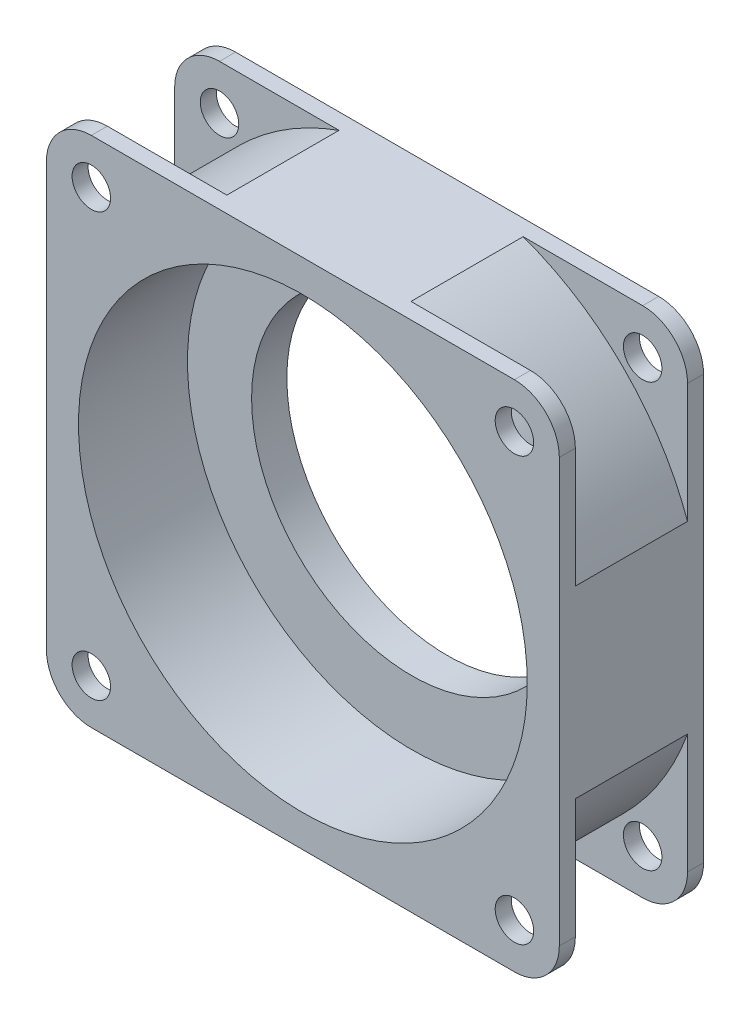
ISO-10303-21;
HEADER;
FILE_DESCRIPTION(('STEP AP214'),'2;1');
FILE_NAME('part.step','',(''),(''),'','','');
FILE_SCHEMA(('AUTOMOTIVE_DESIGN { 1 0 10303 214 1 1 1 1 }'));
ENDSEC;
DATA;
#1=APPLICATION_CONTEXT('core data for automotive mechanical design processes');
#2=APPLICATION_PROTOCOL_DEFINITION('international standard','automotive_design',2000,#1);
#3=PRODUCT_CONTEXT('',#1,'mechanical');
#4=PRODUCT('Part','Part','',(#3));
#5=PRODUCT_RELATED_PRODUCT_CATEGORY('part','',(#4));
#6=PRODUCT_DEFINITION_FORMATION('','',#4);
#7=PRODUCT_DEFINITION_CONTEXT('part definition',#1,'design');
#8=PRODUCT_DEFINITION('design','',#6,#7);
#9=PRODUCT_DEFINITION_SHAPE('','',#8);
#10=(LENGTH_UNIT() NAMED_UNIT(*) SI_UNIT(.MILLI.,.METRE.));
#11=(NAMED_UNIT(*) PLANE_ANGLE_UNIT() SI_UNIT($,.RADIAN.));
#12=(NAMED_UNIT(*) SI_UNIT($,.STERADIAN.) SOLID_ANGLE_UNIT());
#13=UNCERTAINTY_MEASURE_WITH_UNIT(LENGTH_MEASURE(1.E-05),#10,'distance_accuracy_value','');
#14=(GEOMETRIC_REPRESENTATION_CONTEXT(3) GLOBAL_UNCERTAINTY_ASSIGNED_CONTEXT((#13)) GLOBAL_UNIT_ASSIGNED_CONTEXT((#10,
#11,#12)) REPRESENTATION_CONTEXT('',''));
#15=CARTESIAN_POINT('',(0.,0.,0.));
#16=DIRECTION('',(0.,0.,1.));
#17=DIRECTION('',(1.,0.,0.));
#18=AXIS2_PLACEMENT_3D('',#15,#16,#17);
#19=CARTESIAN_POINT('',(0.,0.,20.));
#20=DIRECTION('',(0.,0.,1.));
#21=DIRECTION('',(1.,0.,0.));
#22=AXIS2_PLACEMENT_3D('',#19,#20,#21);
#23=PLANE('',#22);
#24=CARTESIAN_POINT('',(-33.,73.,20.));
#25=DIRECTION('',(0.,0.,1.));
#26=DIRECTION('',(1.,0.,0.));
#27=AXIS2_PLACEMENT_3D('',#24,#25,#26);
#28=CIRCLE('',#27,3.);
#29=CARTESIAN_POINT('',(-30.,73.,20.));
#30=VERTEX_POINT('',#29);
#31=EDGE_CURVE('E381',#30,#30,#28,.T.);
#32=ORIENTED_EDGE('',*,*,#31,.T.);
#33=EDGE_LOOP('',(#32));
#34=FACE_BOUND('',#33,.T.);
#35=DIRECTION('',(-1.,0.,0.));
#36=VECTOR('',#35,1.);
#37=CARTESIAN_POINT('',(0.,80.,20.));
#38=LINE('',#37,#36);
#39=CARTESIAN_POINT('',(-14.3614066163451,80.,20.));
#40=VERTEX_POINT('',#39);
#41=CARTESIAN_POINT('',(-33.,80.,20.));
#42=VERTEX_POINT('',#41);
#43=EDGE_CURVE('E262',#40,#42,#38,.T.);
#44=ORIENTED_EDGE('',*,*,#43,.F.);
#45=CARTESIAN_POINT('',(0.,40.,20.));
#46=DIRECTION('',(0.,0.,1.));
#47=DIRECTION('',(1.,0.,0.));
#48=AXIS2_PLACEMENT_3D('',#45,#46,#47);
#49=CIRCLE('',#48,42.5);
#50=CARTESIAN_POINT('',(-40.,54.3614066163451,20.));
#51=VERTEX_POINT('',#50);
#52=EDGE_CURVE('E249',#40,#51,#49,.T.);
#53=ORIENTED_EDGE('',*,*,#52,.T.);
#54=DIRECTION('',(0.,-1.,0.));
#55=VECTOR('',#54,1.);
#56=CARTESIAN_POINT('',(-40.,0.,20.));
#57=LINE('',#56,#55);
#58=CARTESIAN_POINT('',(-40.,72.9999999999999,20.));
#59=VERTEX_POINT('',#58);
#60=EDGE_CURVE('E268',#59,#51,#57,.T.);
#61=ORIENTED_EDGE('',*,*,#60,.F.);
#62=CARTESIAN_POINT('',(-33.,73.,20.));
#63=DIRECTION('',(0.,0.,1.));
#64=DIRECTION('',(1.,0.,0.));
#65=AXIS2_PLACEMENT_3D('',#62,#63,#64);
#66=CIRCLE('',#65,7.);
#67=EDGE_CURVE('E263',#42,#59,#66,.T.);
#68=ORIENTED_EDGE('',*,*,#67,.F.);
#69=EDGE_LOOP('',(#44,#53,#61,#68));
#70=FACE_BOUND('',#69,.T.);
#71=ADVANCED_FACE('F50',(#34,#70),#23,.F.);
#72=CARTESIAN_POINT('',(33.,73.,20.));
#73=DIRECTION('',(0.,0.,1.));
#74=DIRECTION('',(1.,0.,0.));
#75=AXIS2_PLACEMENT_3D('',#72,#73,#74);
#76=CIRCLE('',#75,3.00000000000001);
#77=CARTESIAN_POINT('',(36.,73.,20.));
#78=VERTEX_POINT('',#77);
#79=EDGE_CURVE('E389',#78,#78,#76,.T.);
#80=ORIENTED_EDGE('',*,*,#79,.T.);
#81=EDGE_LOOP('',(#80));
#82=FACE_BOUND('',#81,.T.);
#83=DIRECTION('',(0.,1.,0.));
#84=VECTOR('',#83,1.);
#85=CARTESIAN_POINT('',(40.,0.,20.));
#86=LINE('',#85,#84);
#87=CARTESIAN_POINT('',(40.,54.3614066163451,20.));
#88=VERTEX_POINT('',#87);
#89=CARTESIAN_POINT('',(40.,72.9999999999999,20.));
#90=VERTEX_POINT('',#89);
#91=EDGE_CURVE('E259',#88,#90,#86,.T.);
#92=ORIENTED_EDGE('',*,*,#91,.F.);
#93=CARTESIAN_POINT('',(0.,40.,20.));
#94=DIRECTION('',(0.,0.,1.));
#95=DIRECTION('',(1.,0.,0.));
#96=AXIS2_PLACEMENT_3D('',#93,#94,#95);
#97=CIRCLE('',#96,42.5);
#98=CARTESIAN_POINT('',(14.3614066163451,80.,20.));
#99=VERTEX_POINT('',#98);
#100=EDGE_CURVE('E250',#88,#99,#97,.T.);
#101=ORIENTED_EDGE('',*,*,#100,.T.);
#102=CARTESIAN_POINT('',(33.,80.,20.));
#103=VERTEX_POINT('',#102);
#104=EDGE_CURVE('E265',#103,#99,#38,.T.);
#105=ORIENTED_EDGE('',*,*,#104,.F.);
#106=CARTESIAN_POINT('',(33.,73.,20.));
#107=DIRECTION('',(0.,0.,1.));
#108=DIRECTION('',(1.,0.,0.));
#109=AXIS2_PLACEMENT_3D('',#106,#107,#108);
#110=CIRCLE('',#109,7.);
#111=EDGE_CURVE('E260',#90,#103,#110,.T.);
#112=ORIENTED_EDGE('',*,*,#111,.F.);
#113=EDGE_LOOP('',(#92,#101,#105,#112));
#114=FACE_BOUND('',#113,.T.);
#115=ADVANCED_FACE('F494',(#82,#114),#23,.F.);
#116=CARTESIAN_POINT('',(33.,7.,20.));
#117=DIRECTION('',(0.,0.,1.));
#118=DIRECTION('',(1.,0.,0.));
#119=AXIS2_PLACEMENT_3D('',#116,#117,#118);
#120=CIRCLE('',#119,3.);
#121=CARTESIAN_POINT('',(36.,7.,20.));
#122=VERTEX_POINT('',#121);
#123=EDGE_CURVE('E395',#122,#122,#120,.T.);
#124=ORIENTED_EDGE('',*,*,#123,.T.);
#125=EDGE_LOOP('',(#124));
#126=FACE_BOUND('',#125,.T.);
#127=DIRECTION('',(1.,0.,0.));
#128=VECTOR('',#127,1.);
#129=CARTESIAN_POINT('',(0.,0.,20.));
#130=LINE('',#129,#128);
#131=CARTESIAN_POINT('',(14.3614066163451,0.,20.));
#132=VERTEX_POINT('',#131);
#133=CARTESIAN_POINT('',(33.,0.,20.));
#134=VERTEX_POINT('',#133);
#135=EDGE_CURVE('E273',#132,#134,#130,.T.);
#136=ORIENTED_EDGE('',*,*,#135,.F.);
#137=CARTESIAN_POINT('',(0.,40.,20.));
#138=DIRECTION('',(0.,0.,1.));
#139=DIRECTION('',(1.,0.,0.));
#140=AXIS2_PLACEMENT_3D('',#137,#138,#139);
#141=CIRCLE('',#140,42.5);
#142=CARTESIAN_POINT('',(40.,25.6385933836549,20.));
#143=VERTEX_POINT('',#142);
#144=EDGE_CURVE('E243',#132,#143,#141,.T.);
#145=ORIENTED_EDGE('',*,*,#144,.T.);
#146=CARTESIAN_POINT('',(40.,7.00000000000005,20.));
#147=VERTEX_POINT('',#146);
#148=EDGE_CURVE('E251',#147,#143,#86,.T.);
#149=ORIENTED_EDGE('',*,*,#148,.F.);
#150=CARTESIAN_POINT('',(33.,7.,20.));
#151=DIRECTION('',(0.,0.,1.));
#152=DIRECTION('',(1.,0.,0.));
#153=AXIS2_PLACEMENT_3D('',#150,#151,#152);
#154=CIRCLE('',#153,7.);
#155=EDGE_CURVE('E276',#134,#147,#154,.T.);
#156=ORIENTED_EDGE('',*,*,#155,.F.);
#157=EDGE_LOOP('',(#136,#145,#149,#156));
#158=FACE_BOUND('',#157,.T.);
#159=ADVANCED_FACE('F439',(#126,#158),#23,.F.);
#160=CARTESIAN_POINT('',(33.,7.,20.));
#161=DIRECTION('',(0.,0.,1.));
#162=DIRECTION('',(1.,0.,0.));
#163=AXIS2_PLACEMENT_3D('',#160,#161,#162);
#164=CYLINDRICAL_SURFACE('',#163,7.);
#165=CARTESIAN_POINT('',(33.,7.,22.5));
#166=DIRECTION('',(0.,0.,1.));
#167=DIRECTION('',(1.,0.,0.));
#168=AXIS2_PLACEMENT_3D('',#165,#166,#167);
#169=CIRCLE('',#168,7.);
#170=CARTESIAN_POINT('',(33.,0.,22.5));
#171=VERTEX_POINT('',#170);
#172=CARTESIAN_POINT('',(40.,7.00000000000005,22.5));
#173=VERTEX_POINT('',#172);
#174=EDGE_CURVE('E299',#171,#173,#169,.T.);
#175=ORIENTED_EDGE('',*,*,#174,.F.);
#176=DIRECTION('',(0.,0.,1.));
#177=VECTOR('',#176,1.);
#178=CARTESIAN_POINT('',(33.,0.,20.));
#179=LINE('',#178,#177);
#180=EDGE_CURVE('E304',#134,#171,#179,.T.);
#181=ORIENTED_EDGE('',*,*,#180,.F.);
#182=ORIENTED_EDGE('',*,*,#155,.T.);
#183=DIRECTION('',(0.,0.,1.));
#184=VECTOR('',#183,1.);
#185=CARTESIAN_POINT('',(40.,7.00000000000005,20.));
#186=LINE('',#185,#184);
#187=EDGE_CURVE('E305',#147,#173,#186,.T.);
#188=ORIENTED_EDGE('',*,*,#187,.T.);
#189=EDGE_LOOP('',(#175,#181,#182,#188));
#190=FACE_BOUND('',#189,.T.);
#191=ADVANCED_FACE('F443',(#190),#164,.T.);
#192=CARTESIAN_POINT('',(-33.,7.,20.));
#193=DIRECTION('',(0.,0.,1.));
#194=DIRECTION('',(1.,0.,0.));
#195=AXIS2_PLACEMENT_3D('',#192,#193,#194);
#196=CYLINDRICAL_SURFACE('',#195,7.);
#197=CARTESIAN_POINT('',(-33.,7.,22.5));
#198=DIRECTION('',(0.,0.,1.));
#199=DIRECTION('',(1.,0.,0.));
#200=AXIS2_PLACEMENT_3D('',#197,#198,#199);
#201=CIRCLE('',#200,7.);
#202=CARTESIAN_POINT('',(-33.,0.,22.5));
#203=VERTEX_POINT('',#202);
#204=CARTESIAN_POINT('',(-40.,7.00000000000005,22.5));
#205=VERTEX_POINT('',#204);
#206=EDGE_CURVE('E295',#203,#205,#201,.F.);
#207=ORIENTED_EDGE('',*,*,#206,.T.);
#208=DIRECTION('',(0.,0.,1.));
#209=VECTOR('',#208,1.);
#210=CARTESIAN_POINT('',(-40.,7.00000000000005,20.));
#211=LINE('',#210,#209);
#212=CARTESIAN_POINT('',(-40.,7.00000000000005,20.));
#213=VERTEX_POINT('',#212);
#214=EDGE_CURVE('E309',#213,#205,#211,.T.);
#215=ORIENTED_EDGE('',*,*,#214,.F.);
#216=CARTESIAN_POINT('',(-33.,7.,20.));
#217=DIRECTION('',(0.,0.,1.));
#218=DIRECTION('',(1.,0.,0.));
#219=AXIS2_PLACEMENT_3D('',#216,#217,#218);
#220=CIRCLE('',#219,7.);
#221=CARTESIAN_POINT('',(-33.,0.,20.));
#222=VERTEX_POINT('',#221);
#223=EDGE_CURVE('E275',#222,#213,#220,.F.);
#224=ORIENTED_EDGE('',*,*,#223,.F.);
#225=DIRECTION('',(0.,0.,1.));
#226=VECTOR('',#225,1.);
#227=CARTESIAN_POINT('',(-33.,0.,20.));
#228=LINE('',#227,#226);
#229=EDGE_CURVE('E308',#222,#203,#228,.T.);
#230=ORIENTED_EDGE('',*,*,#229,.T.);
#231=EDGE_LOOP('',(#207,#215,#224,#230));
#232=FACE_BOUND('',#231,.T.);
#233=ADVANCED_FACE('F451',(#232),#196,.T.);
#234=CARTESIAN_POINT('',(-33.,73.,20.));
#235=DIRECTION('',(0.,0.,1.));
#236=DIRECTION('',(1.,0.,0.));
#237=AXIS2_PLACEMENT_3D('',#234,#235,#236);
#238=CYLINDRICAL_SURFACE('',#237,7.);
#239=CARTESIAN_POINT('',(-33.,73.,22.5));
#240=DIRECTION('',(0.,0.,1.));
#241=DIRECTION('',(1.,0.,0.));
#242=AXIS2_PLACEMENT_3D('',#239,#240,#241);
#243=CIRCLE('',#242,7.);
#244=CARTESIAN_POINT('',(-33.,80.,22.5));
#245=VERTEX_POINT('',#244);
#246=CARTESIAN_POINT('',(-40.,72.9999999999999,22.5));
#247=VERTEX_POINT('',#246);
#248=EDGE_CURVE('E288',#245,#247,#243,.T.);
#249=ORIENTED_EDGE('',*,*,#248,.F.);
#250=DIRECTION('',(0.,0.,1.));
#251=VECTOR('',#250,1.);
#252=CARTESIAN_POINT('',(-33.,80.,20.));
#253=LINE('',#252,#251);
#254=EDGE_CURVE('E314',#42,#245,#253,.T.);
#255=ORIENTED_EDGE('',*,*,#254,.F.);
#256=ORIENTED_EDGE('',*,*,#67,.T.);
#257=DIRECTION('',(0.,0.,1.));
#258=VECTOR('',#257,1.);
#259=CARTESIAN_POINT('',(-40.,72.9999999999999,20.));
#260=LINE('',#259,#258);
#261=EDGE_CURVE('E312',#59,#247,#260,.T.);
#262=ORIENTED_EDGE('',*,*,#261,.T.);
#263=EDGE_LOOP('',(#249,#255,#256,#262));
#264=FACE_BOUND('',#263,.T.);
#265=ADVANCED_FACE('F517',(#264),#238,.T.);
#266=CARTESIAN_POINT('',(33.,73.,20.));
#267=DIRECTION('',(0.,0.,1.));
#268=DIRECTION('',(1.,0.,0.));
#269=AXIS2_PLACEMENT_3D('',#266,#267,#268);
#270=CYLINDRICAL_SURFACE('',#269,7.);
#271=CARTESIAN_POINT('',(33.,73.,22.5));
#272=DIRECTION('',(0.,0.,1.));
#273=DIRECTION('',(1.,0.,0.));
#274=AXIS2_PLACEMENT_3D('',#271,#272,#273);
#275=CIRCLE('',#274,7.);
#276=CARTESIAN_POINT('',(40.,72.9999999999999,22.5));
#277=VERTEX_POINT('',#276);
#278=CARTESIAN_POINT('',(33.,80.,22.5));
#279=VERTEX_POINT('',#278);
#280=EDGE_CURVE('E281',#277,#279,#275,.T.);
#281=ORIENTED_EDGE('',*,*,#280,.F.);
#282=DIRECTION('',(0.,0.,1.));
#283=VECTOR('',#282,1.);
#284=CARTESIAN_POINT('',(40.,72.9999999999999,20.));
#285=LINE('',#284,#283);
#286=EDGE_CURVE('E285',#90,#277,#285,.T.);
#287=ORIENTED_EDGE('',*,*,#286,.F.);
#288=ORIENTED_EDGE('',*,*,#111,.T.);
#289=DIRECTION('',(0.,0.,1.));
#290=VECTOR('',#289,1.);
#291=CARTESIAN_POINT('',(33.,80.,20.));
#292=LINE('',#291,#290);
#293=EDGE_CURVE('E319',#103,#279,#292,.T.);
#294=ORIENTED_EDGE('',*,*,#293,.T.);
#295=EDGE_LOOP('',(#281,#287,#288,#294));
#296=FACE_BOUND('',#295,.T.);
#297=ADVANCED_FACE('F506',(#296),#270,.T.);
#298=CARTESIAN_POINT('',(-33.,7.,20.));
#299=DIRECTION('',(0.,0.,1.));
#300=DIRECTION('',(1.,0.,0.));
#301=AXIS2_PLACEMENT_3D('',#298,#299,#300);
#302=CIRCLE('',#301,3.);
#303=CARTESIAN_POINT('',(-30.,7.,20.));
#304=VERTEX_POINT('',#303);
#305=EDGE_CURVE('E410',#304,#304,#302,.T.);
#306=ORIENTED_EDGE('',*,*,#305,.T.);
#307=EDGE_LOOP('',(#306));
#308=FACE_BOUND('',#307,.T.);
#309=CARTESIAN_POINT('',(-40.,25.6385933836549,20.));
#310=VERTEX_POINT('',#309);
#311=EDGE_CURVE('E267',#310,#213,#57,.T.);
#312=ORIENTED_EDGE('',*,*,#311,.F.);
#313=CARTESIAN_POINT('',(0.,40.,20.));
#314=DIRECTION('',(0.,0.,1.));
#315=DIRECTION('',(1.,0.,0.));
#316=AXIS2_PLACEMENT_3D('',#313,#314,#315);
#317=CIRCLE('',#316,42.5);
#318=CARTESIAN_POINT('',(-14.3614066163451,0.,20.));
#319=VERTEX_POINT('',#318);
#320=EDGE_CURVE('E233',#310,#319,#317,.T.);
#321=ORIENTED_EDGE('',*,*,#320,.T.);
#322=EDGE_CURVE('E277',#222,#319,#130,.T.);
#323=ORIENTED_EDGE('',*,*,#322,.F.);
#324=ORIENTED_EDGE('',*,*,#223,.T.);
#325=EDGE_LOOP('',(#312,#321,#323,#324));
#326=FACE_BOUND('',#325,.T.);
#327=ADVANCED_FACE('F460',(#308,#326),#23,.F.);
#328=CARTESIAN_POINT('',(0.,40.,22.5));
#329=DIRECTION('',(0.,0.,1.));
#330=DIRECTION('',(1.,0.,0.));
#331=AXIS2_PLACEMENT_3D('',#328,#329,#330);
#332=PLANE('',#331);
#333=CARTESIAN_POINT('',(33.,73.,22.5));
#334=DIRECTION('',(0.,0.,1.));
#335=DIRECTION('',(1.,0.,0.));
#336=AXIS2_PLACEMENT_3D('',#333,#334,#335);
#337=CIRCLE('',#336,3.00000000000001);
#338=CARTESIAN_POINT('',(36.,73.,22.5));
#339=VERTEX_POINT('',#338);
#340=EDGE_CURVE('E880',#339,#339,#337,.T.);
#341=ORIENTED_EDGE('',*,*,#340,.F.);
#342=EDGE_LOOP('',(#341));
#343=FACE_BOUND('',#342,.T.);
#344=CARTESIAN_POINT('',(-33.,7.,22.5));
#345=DIRECTION('',(0.,0.,1.));
#346=DIRECTION('',(1.,0.,0.));
#347=AXIS2_PLACEMENT_3D('',#344,#345,#346);
#348=CIRCLE('',#347,3.);
#349=CARTESIAN_POINT('',(-30.,7.,22.5));
#350=VERTEX_POINT('',#349);
#351=EDGE_CURVE('E879',#350,#350,#348,.T.);
#352=ORIENTED_EDGE('',*,*,#351,.F.);
#353=EDGE_LOOP('',(#352));
#354=FACE_BOUND('',#353,.T.);
#355=CARTESIAN_POINT('',(33.,7.,22.5));
#356=DIRECTION('',(0.,0.,1.));
#357=DIRECTION('',(1.,0.,0.));
#358=AXIS2_PLACEMENT_3D('',#355,#356,#357);
#359=CIRCLE('',#358,3.);
#360=CARTESIAN_POINT('',(36.,7.,22.5));
#361=VERTEX_POINT('',#360);
#362=EDGE_CURVE('E882',#361,#361,#359,.T.);
#363=ORIENTED_EDGE('',*,*,#362,.F.);
#364=EDGE_LOOP('',(#363));
#365=FACE_BOUND('',#364,.T.);
#366=CARTESIAN_POINT('',(-33.,73.,22.5));
#367=DIRECTION('',(0.,0.,1.));
#368=DIRECTION('',(1.,0.,0.));
#369=AXIS2_PLACEMENT_3D('',#366,#367,#368);
#370=CIRCLE('',#369,3.);
#371=CARTESIAN_POINT('',(-30.,73.,22.5));
#372=VERTEX_POINT('',#371);
#373=EDGE_CURVE('E379',#372,#372,#370,.T.);
#374=ORIENTED_EDGE('',*,*,#373,.F.);
#375=EDGE_LOOP('',(#374));
#376=FACE_BOUND('',#375,.T.);
#377=CARTESIAN_POINT('',(0.,40.,22.5));
#378=DIRECTION('',(0.,0.,1.));
#379=DIRECTION('',(1.,0.,0.));
#380=AXIS2_PLACEMENT_3D('',#377,#378,#379);
#381=CIRCLE('',#380,35.);
#382=CARTESIAN_POINT('',(35.,40.,22.5));
#383=VERTEX_POINT('',#382);
#384=EDGE_CURVE('E372',#383,#383,#381,.T.);
#385=ORIENTED_EDGE('',*,*,#384,.F.);
#386=EDGE_LOOP('',(#385));
#387=FACE_BOUND('',#386,.T.);
#388=DIRECTION('',(1.,0.,0.));
#389=VECTOR('',#388,1.);
#390=CARTESIAN_POINT('',(0.,0.,22.5));
#391=LINE('',#390,#389);
#392=EDGE_CURVE('E300',#203,#171,#391,.T.);
#393=ORIENTED_EDGE('',*,*,#392,.T.);
#394=ORIENTED_EDGE('',*,*,#174,.T.);
#395=DIRECTION('',(0.,1.,0.));
#396=VECTOR('',#395,1.);
#397=CARTESIAN_POINT('',(40.,0.,22.5));
#398=LINE('',#397,#396);
#399=EDGE_CURVE('E254',#173,#277,#398,.T.);
#400=ORIENTED_EDGE('',*,*,#399,.T.);
#401=ORIENTED_EDGE('',*,*,#280,.T.);
#402=DIRECTION('',(-1.,0.,0.));
#403=VECTOR('',#402,1.);
#404=CARTESIAN_POINT('',(0.,80.,22.5));
#405=LINE('',#404,#403);
#406=EDGE_CURVE('E290',#279,#245,#405,.T.);
#407=ORIENTED_EDGE('',*,*,#406,.T.);
#408=ORIENTED_EDGE('',*,*,#248,.T.);
#409=DIRECTION('',(0.,-1.,0.));
#410=VECTOR('',#409,1.);
#411=CARTESIAN_POINT('',(-40.,0.,22.5));
#412=LINE('',#411,#410);
#413=EDGE_CURVE('E292',#247,#205,#412,.T.);
#414=ORIENTED_EDGE('',*,*,#413,.T.);
#415=ORIENTED_EDGE('',*,*,#206,.F.);
#416=EDGE_LOOP('',(#393,#394,#400,#401,#407,#408,#414,#415));
#417=FACE_BOUND('',#416,.T.);
#418=ADVANCED_FACE('F448',(#343,#354,#365,#376,#387,#417),#332,.T.);
#419=CARTESIAN_POINT('',(0.,40.,2.5));
#420=DIRECTION('',(0.,0.,1.));
#421=DIRECTION('',(1.,0.,0.));
#422=AXIS2_PLACEMENT_3D('',#419,#420,#421);
#423=CYLINDRICAL_SURFACE('',#422,42.5);
#424=ORIENTED_EDGE('',*,*,#52,.F.);
#425=DIRECTION('',(0.,0.,1.));
#426=VECTOR('',#425,1.);
#427=CARTESIAN_POINT('',(-14.3614066163451,80.,2.5));
#428=LINE('',#427,#426);
#429=CARTESIAN_POINT('',(-14.3614066163451,80.,2.5));
#430=VERTEX_POINT('',#429);
#431=EDGE_CURVE('E242',#430,#40,#428,.T.);
#432=ORIENTED_EDGE('',*,*,#431,.F.);
#433=CARTESIAN_POINT('',(0.,40.,2.5));
#434=DIRECTION('',(0.,0.,1.));
#435=DIRECTION('',(1.,0.,0.));
#436=AXIS2_PLACEMENT_3D('',#433,#434,#435);
#437=CIRCLE('',#436,42.5);
#438=CARTESIAN_POINT('',(-40.,54.3614066163451,2.5));
#439=VERTEX_POINT('',#438);
#440=EDGE_CURVE('E66',#430,#439,#437,.T.);
#441=ORIENTED_EDGE('',*,*,#440,.T.);
#442=DIRECTION('',(0.,0.,1.));
#443=VECTOR('',#442,1.);
#444=CARTESIAN_POINT('',(-40.,54.3614066163451,2.5));
#445=LINE('',#444,#443);
#446=EDGE_CURVE('E234',#439,#51,#445,.T.);
#447=ORIENTED_EDGE('',*,*,#446,.T.);
#448=EDGE_LOOP('',(#424,#432,#441,#447));
#449=FACE_BOUND('',#448,.T.);
#450=ADVANCED_FACE('F489',(#449),#423,.T.);
#451=CARTESIAN_POINT('',(0.,40.,2.5));
#452=DIRECTION('',(0.,0.,1.));
#453=DIRECTION('',(1.,0.,0.));
#454=AXIS2_PLACEMENT_3D('',#451,#452,#453);
#455=CYLINDRICAL_SURFACE('',#454,42.5);
#456=ORIENTED_EDGE('',*,*,#100,.F.);
#457=DIRECTION('',(0.,0.,1.));
#458=VECTOR('',#457,1.);
#459=CARTESIAN_POINT('',(40.,54.3614066163451,2.5));
#460=LINE('',#459,#458);
#461=CARTESIAN_POINT('',(40.,54.3614066163451,2.5));
#462=VERTEX_POINT('',#461);
#463=EDGE_CURVE('E428',#462,#88,#460,.T.);
#464=ORIENTED_EDGE('',*,*,#463,.F.);
#465=CARTESIAN_POINT('',(0.,40.,2.5));
#466=DIRECTION('',(0.,0.,1.));
#467=DIRECTION('',(1.,0.,0.));
#468=AXIS2_PLACEMENT_3D('',#465,#466,#467);
#469=CIRCLE('',#468,42.5);
#470=CARTESIAN_POINT('',(14.3614066163451,80.,2.5));
#471=VERTEX_POINT('',#470);
#472=EDGE_CURVE('E238',#462,#471,#469,.T.);
#473=ORIENTED_EDGE('',*,*,#472,.T.);
#474=DIRECTION('',(0.,0.,1.));
#475=VECTOR('',#474,1.);
#476=CARTESIAN_POINT('',(14.3614066163451,80.,2.5));
#477=LINE('',#476,#475);
#478=EDGE_CURVE('E425',#471,#99,#477,.T.);
#479=ORIENTED_EDGE('',*,*,#478,.T.);
#480=EDGE_LOOP('',(#456,#464,#473,#479));
#481=FACE_BOUND('',#480,.T.);
#482=ADVANCED_FACE('F485',(#481),#455,.T.);
#483=CARTESIAN_POINT('',(0.,40.,2.5));
#484=DIRECTION('',(0.,0.,1.));
#485=DIRECTION('',(1.,0.,0.));
#486=AXIS2_PLACEMENT_3D('',#483,#484,#485);
#487=CYLINDRICAL_SURFACE('',#486,42.5);
#488=ORIENTED_EDGE('',*,*,#144,.F.);
#489=DIRECTION('',(0.,0.,1.));
#490=VECTOR('',#489,1.);
#491=CARTESIAN_POINT('',(14.3614066163451,0.,2.5));
#492=LINE('',#491,#490);
#493=CARTESIAN_POINT('',(14.3614066163451,0.,2.5));
#494=VERTEX_POINT('',#493);
#495=EDGE_CURVE('E236',#494,#132,#492,.T.);
#496=ORIENTED_EDGE('',*,*,#495,.F.);
#497=CARTESIAN_POINT('',(0.,40.,2.5));
#498=DIRECTION('',(0.,0.,1.));
#499=DIRECTION('',(1.,0.,0.));
#500=AXIS2_PLACEMENT_3D('',#497,#498,#499);
#501=CIRCLE('',#500,42.5);
#502=CARTESIAN_POINT('',(40.,25.6385933836549,2.5));
#503=VERTEX_POINT('',#502);
#504=EDGE_CURVE('E227',#494,#503,#501,.T.);
#505=ORIENTED_EDGE('',*,*,#504,.T.);
#506=DIRECTION('',(0.,0.,1.));
#507=VECTOR('',#506,1.);
#508=CARTESIAN_POINT('',(40.,25.6385933836549,2.5));
#509=LINE('',#508,#507);
#510=EDGE_CURVE('E429',#503,#143,#509,.T.);
#511=ORIENTED_EDGE('',*,*,#510,.T.);
#512=EDGE_LOOP('',(#488,#496,#505,#511));
#513=FACE_BOUND('',#512,.T.);
#514=ADVANCED_FACE('F478',(#513),#487,.T.);
#515=CARTESIAN_POINT('',(0.,40.,2.5));
#516=DIRECTION('',(0.,0.,1.));
#517=DIRECTION('',(1.,0.,0.));
#518=AXIS2_PLACEMENT_3D('',#515,#516,#517);
#519=CYLINDRICAL_SURFACE('',#518,42.5);
#520=ORIENTED_EDGE('',*,*,#320,.F.);
#521=DIRECTION('',(0.,0.,1.));
#522=VECTOR('',#521,1.);
#523=CARTESIAN_POINT('',(-40.,25.6385933836549,2.5));
#524=LINE('',#523,#522);
#525=CARTESIAN_POINT('',(-40.,25.6385933836549,2.5));
#526=VERTEX_POINT('',#525);
#527=EDGE_CURVE('E215',#526,#310,#524,.T.);
#528=ORIENTED_EDGE('',*,*,#527,.F.);
#529=CARTESIAN_POINT('',(0.,40.,2.5));
#530=DIRECTION('',(0.,0.,1.));
#531=DIRECTION('',(1.,0.,0.));
#532=AXIS2_PLACEMENT_3D('',#529,#530,#531);
#533=CIRCLE('',#532,42.5);
#534=CARTESIAN_POINT('',(-14.3614066163451,0.,2.5));
#535=VERTEX_POINT('',#534);
#536=EDGE_CURVE('E221',#526,#535,#533,.T.);
#537=ORIENTED_EDGE('',*,*,#536,.T.);
#538=DIRECTION('',(0.,0.,1.));
#539=VECTOR('',#538,1.);
#540=CARTESIAN_POINT('',(-14.3614066163451,0.,2.5));
#541=LINE('',#540,#539);
#542=EDGE_CURVE('E231',#535,#319,#541,.T.);
#543=ORIENTED_EDGE('',*,*,#542,.T.);
#544=EDGE_LOOP('',(#520,#528,#537,#543));
#545=FACE_BOUND('',#544,.T.);
#546=ADVANCED_FACE('F230',(#545),#519,.T.);
#547=CARTESIAN_POINT('',(33.,73.,2.5));
#548=DIRECTION('',(0.,0.,-1.));
#549=DIRECTION('',(-1.,0.,0.));
#550=AXIS2_PLACEMENT_3D('',#547,#548,#549);
#551=CYLINDRICAL_SURFACE('',#550,7.);
#552=CARTESIAN_POINT('',(33.,73.,0.));
#553=DIRECTION('',(0.,0.,1.));
#554=DIRECTION('',(1.,0.,0.));
#555=AXIS2_PLACEMENT_3D('',#552,#553,#554);
#556=CIRCLE('',#555,7.);
#557=CARTESIAN_POINT('',(40.,73.,0.));
#558=VERTEX_POINT('',#557);
#559=CARTESIAN_POINT('',(33.,80.,0.));
#560=VERTEX_POINT('',#559);
#561=EDGE_CURVE('E344',#558,#560,#556,.T.);
#562=ORIENTED_EDGE('',*,*,#561,.T.);
#563=DIRECTION('',(0.,0.,-1.));
#564=VECTOR('',#563,1.);
#565=CARTESIAN_POINT('',(33.,80.,2.5));
#566=LINE('',#565,#564);
#567=CARTESIAN_POINT('',(33.,80.,2.5));
#568=VERTEX_POINT('',#567);
#569=EDGE_CURVE('E361',#568,#560,#566,.T.);
#570=ORIENTED_EDGE('',*,*,#569,.F.);
#571=CARTESIAN_POINT('',(33.,73.,2.5));
#572=DIRECTION('',(0.,0.,1.));
#573=DIRECTION('',(1.,0.,0.));
#574=AXIS2_PLACEMENT_3D('',#571,#572,#573);
#575=CIRCLE('',#574,7.);
#576=CARTESIAN_POINT('',(40.,73.,2.5));
#577=VERTEX_POINT('',#576);
#578=EDGE_CURVE('E326',#577,#568,#575,.T.);
#579=ORIENTED_EDGE('',*,*,#578,.F.);
#580=DIRECTION('',(0.,0.,-1.));
#581=VECTOR('',#580,1.);
#582=CARTESIAN_POINT('',(40.,73.,2.5));
#583=LINE('',#582,#581);
#584=EDGE_CURVE('E366',#577,#558,#583,.T.);
#585=ORIENTED_EDGE('',*,*,#584,.T.);
#586=EDGE_LOOP('',(#562,#570,#579,#585));
#587=FACE_BOUND('',#586,.T.);
#588=ADVANCED_FACE('F486',(#587),#551,.T.);
#589=CARTESIAN_POINT('',(33.,7.,2.5));
#590=DIRECTION('',(0.,0.,-1.));
#591=DIRECTION('',(-1.,0.,0.));
#592=AXIS2_PLACEMENT_3D('',#589,#590,#591);
#593=CYLINDRICAL_SURFACE('',#592,7.);
#594=CARTESIAN_POINT('',(33.,7.,0.));
#595=DIRECTION('',(0.,0.,1.));
#596=DIRECTION('',(1.,0.,0.));
#597=AXIS2_PLACEMENT_3D('',#594,#595,#596);
#598=CIRCLE('',#597,7.);
#599=CARTESIAN_POINT('',(33.,0.,0.));
#600=VERTEX_POINT('',#599);
#601=CARTESIAN_POINT('',(40.,7.,0.));
#602=VERTEX_POINT('',#601);
#603=EDGE_CURVE('E339',#600,#602,#598,.T.);
#604=ORIENTED_EDGE('',*,*,#603,.T.);
#605=DIRECTION('',(0.,0.,-1.));
#606=VECTOR('',#605,1.);
#607=CARTESIAN_POINT('',(40.,7.,2.5));
#608=LINE('',#607,#606);
#609=CARTESIAN_POINT('',(40.,7.,2.5));
#610=VERTEX_POINT('',#609);
#611=EDGE_CURVE('E57',#610,#602,#608,.T.);
#612=ORIENTED_EDGE('',*,*,#611,.F.);
#613=CARTESIAN_POINT('',(33.,7.,2.5));
#614=DIRECTION('',(0.,0.,1.));
#615=DIRECTION('',(1.,0.,0.));
#616=AXIS2_PLACEMENT_3D('',#613,#614,#615);
#617=CIRCLE('',#616,7.);
#618=CARTESIAN_POINT('',(33.,0.,2.5));
#619=VERTEX_POINT('',#618);
#620=EDGE_CURVE('E324',#619,#610,#617,.T.);
#621=ORIENTED_EDGE('',*,*,#620,.F.);
#622=DIRECTION('',(0.,0.,-1.));
#623=VECTOR('',#622,1.);
#624=CARTESIAN_POINT('',(33.,0.,2.5));
#625=LINE('',#624,#623);
#626=EDGE_CURVE('E11',#619,#600,#625,.T.);
#627=ORIENTED_EDGE('',*,*,#626,.T.);
#628=EDGE_LOOP('',(#604,#612,#621,#627));
#629=FACE_BOUND('',#628,.T.);
#630=ADVANCED_FACE('F472',(#629),#593,.T.);
#631=CARTESIAN_POINT('',(-33.,73.,2.5));
#632=DIRECTION('',(0.,0.,-1.));
#633=DIRECTION('',(-1.,0.,0.));
#634=AXIS2_PLACEMENT_3D('',#631,#632,#633);
#635=CYLINDRICAL_SURFACE('',#634,7.);
#636=CARTESIAN_POINT('',(-33.,73.,0.));
#637=DIRECTION('',(0.,0.,1.));
#638=DIRECTION('',(-1.,0.,0.));
#639=AXIS2_PLACEMENT_3D('',#636,#637,#638);
#640=CIRCLE('',#639,7.);
#641=CARTESIAN_POINT('',(-33.,80.,0.));
#642=VERTEX_POINT('',#641);
#643=CARTESIAN_POINT('',(-40.,73.,0.));
#644=VERTEX_POINT('',#643);
#645=EDGE_CURVE('E350',#642,#644,#640,.T.);
#646=ORIENTED_EDGE('',*,*,#645,.T.);
#647=DIRECTION('',(0.,0.,-1.));
#648=VECTOR('',#647,1.);
#649=CARTESIAN_POINT('',(-40.,73.,2.5));
#650=LINE('',#649,#648);
#651=CARTESIAN_POINT('',(-40.,73.,2.5));
#652=VERTEX_POINT('',#651);
#653=EDGE_CURVE('E357',#652,#644,#650,.T.);
#654=ORIENTED_EDGE('',*,*,#653,.F.);
#655=CARTESIAN_POINT('',(-33.,73.,2.5));
#656=DIRECTION('',(0.,0.,1.));
#657=DIRECTION('',(-1.,0.,0.));
#658=AXIS2_PLACEMENT_3D('',#655,#656,#657);
#659=CIRCLE('',#658,7.);
#660=CARTESIAN_POINT('',(-33.,80.,2.5));
#661=VERTEX_POINT('',#660);
#662=EDGE_CURVE('E219',#661,#652,#659,.T.);
#663=ORIENTED_EDGE('',*,*,#662,.F.);
#664=DIRECTION('',(0.,0.,-1.));
#665=VECTOR('',#664,1.);
#666=CARTESIAN_POINT('',(-33.,80.,2.5));
#667=LINE('',#666,#665);
#668=EDGE_CURVE('E359',#661,#642,#667,.T.);
#669=ORIENTED_EDGE('',*,*,#668,.T.);
#670=EDGE_LOOP('',(#646,#654,#663,#669));
#671=FACE_BOUND('',#670,.T.);
#672=ADVANCED_FACE('F625',(#671),#635,.T.);
#673=CARTESIAN_POINT('',(-33.,7.,2.5));
#674=DIRECTION('',(0.,0.,-1.));
#675=DIRECTION('',(-1.,0.,0.));
#676=AXIS2_PLACEMENT_3D('',#673,#674,#675);
#677=CYLINDRICAL_SURFACE('',#676,7.);
#678=CARTESIAN_POINT('',(-33.,7.,0.));
#679=DIRECTION('',(0.,0.,1.));
#680=DIRECTION('',(-1.,0.,0.));
#681=AXIS2_PLACEMENT_3D('',#678,#679,#680);
#682=CIRCLE('',#681,7.);
#683=CARTESIAN_POINT('',(-40.,7.00000000000005,0.));
#684=VERTEX_POINT('',#683);
#685=CARTESIAN_POINT('',(-33.,0.,0.));
#686=VERTEX_POINT('',#685);
#687=EDGE_CURVE('E351',#684,#686,#682,.T.);
#688=ORIENTED_EDGE('',*,*,#687,.T.);
#689=DIRECTION('',(0.,0.,-1.));
#690=VECTOR('',#689,1.);
#691=CARTESIAN_POINT('',(-33.,0.,2.5));
#692=LINE('',#691,#690);
#693=CARTESIAN_POINT('',(-33.,0.,2.5));
#694=VERTEX_POINT('',#693);
#695=EDGE_CURVE('E340',#694,#686,#692,.T.);
#696=ORIENTED_EDGE('',*,*,#695,.F.);
#697=CARTESIAN_POINT('',(-33.,7.,2.5));
#698=DIRECTION('',(0.,0.,1.));
#699=DIRECTION('',(-1.,0.,0.));
#700=AXIS2_PLACEMENT_3D('',#697,#698,#699);
#701=CIRCLE('',#700,7.);
#702=CARTESIAN_POINT('',(-40.,7.00000000000005,2.5));
#703=VERTEX_POINT('',#702);
#704=EDGE_CURVE('E334',#703,#694,#701,.T.);
#705=ORIENTED_EDGE('',*,*,#704,.F.);
#706=DIRECTION('',(0.,0.,-1.));
#707=VECTOR('',#706,1.);
#708=CARTESIAN_POINT('',(-40.,7.00000000000005,2.5));
#709=LINE('',#708,#707);
#710=EDGE_CURVE('E213',#703,#684,#709,.T.);
#711=ORIENTED_EDGE('',*,*,#710,.T.);
#712=EDGE_LOOP('',(#688,#696,#705,#711));
#713=FACE_BOUND('',#712,.T.);
#714=ADVANCED_FACE('F458',(#713),#677,.T.);
#715=CARTESIAN_POINT('',(33.,7.,0.));
#716=DIRECTION('',(0.,0.,1.));
#717=DIRECTION('',(1.,0.,0.));
#718=AXIS2_PLACEMENT_3D('',#715,#716,#717);
#719=PLANE('',#718);
#720=CARTESIAN_POINT('',(33.,73.,0.));
#721=DIRECTION('',(0.,0.,1.));
#722=DIRECTION('',(1.,0.,0.));
#723=AXIS2_PLACEMENT_3D('',#720,#721,#722);
#724=CIRCLE('',#723,3.00000000000001);
#725=CARTESIAN_POINT('',(36.,73.,0.));
#726=VERTEX_POINT('',#725);
#727=EDGE_CURVE('E384',#726,#726,#724,.T.);
#728=ORIENTED_EDGE('',*,*,#727,.T.);
#729=EDGE_LOOP('',(#728));
#730=FACE_BOUND('',#729,.T.);
#731=CARTESIAN_POINT('',(-33.,7.,0.));
#732=DIRECTION('',(0.,0.,1.));
#733=DIRECTION('',(1.,0.,0.));
#734=AXIS2_PLACEMENT_3D('',#731,#732,#733);
#735=CIRCLE('',#734,3.);
#736=CARTESIAN_POINT('',(-30.,7.,0.));
#737=VERTEX_POINT('',#736);
#738=EDGE_CURVE('E404',#737,#737,#735,.T.);
#739=ORIENTED_EDGE('',*,*,#738,.T.);
#740=EDGE_LOOP('',(#739));
#741=FACE_BOUND('',#740,.T.);
#742=CARTESIAN_POINT('',(33.,7.,0.));
#743=DIRECTION('',(0.,0.,1.));
#744=DIRECTION('',(1.,0.,0.));
#745=AXIS2_PLACEMENT_3D('',#742,#743,#744);
#746=CIRCLE('',#745,3.);
#747=CARTESIAN_POINT('',(36.,7.,0.));
#748=VERTEX_POINT('',#747);
#749=EDGE_CURVE('E390',#748,#748,#746,.T.);
#750=ORIENTED_EDGE('',*,*,#749,.T.);
#751=EDGE_LOOP('',(#750));
#752=FACE_BOUND('',#751,.T.);
#753=CARTESIAN_POINT('',(-33.,73.,0.));
#754=DIRECTION('',(0.,0.,1.));
#755=DIRECTION('',(1.,0.,0.));
#756=AXIS2_PLACEMENT_3D('',#753,#754,#755);
#757=CIRCLE('',#756,3.);
#758=CARTESIAN_POINT('',(-30.,73.,0.));
#759=VERTEX_POINT('',#758);
#760=EDGE_CURVE('E378',#759,#759,#757,.T.);
#761=ORIENTED_EDGE('',*,*,#760,.T.);
#762=EDGE_LOOP('',(#761));
#763=FACE_BOUND('',#762,.T.);
#764=CARTESIAN_POINT('',(0.,40.,0.));
#765=DIRECTION('',(0.,0.,1.));
#766=DIRECTION('',(1.,0.,0.));
#767=AXIS2_PLACEMENT_3D('',#764,#765,#766);
#768=CIRCLE('',#767,25.);
#769=CARTESIAN_POINT('',(25.,40.,0.));
#770=VERTEX_POINT('',#769);
#771=EDGE_CURVE('E371',#770,#770,#768,.T.);
#772=ORIENTED_EDGE('',*,*,#771,.T.);
#773=EDGE_LOOP('',(#772));
#774=FACE_BOUND('',#773,.T.);
#775=DIRECTION('',(1.,0.,0.));
#776=VECTOR('',#775,1.);
#777=CARTESIAN_POINT('',(0.,0.,0.));
#778=LINE('',#777,#776);
#779=EDGE_CURVE('E302',#686,#600,#778,.T.);
#780=ORIENTED_EDGE('',*,*,#779,.F.);
#781=ORIENTED_EDGE('',*,*,#687,.F.);
#782=DIRECTION('',(0.,-1.,0.));
#783=VECTOR('',#782,1.);
#784=CARTESIAN_POINT('',(-40.,73.,0.));
#785=LINE('',#784,#783);
#786=EDGE_CURVE('E346',#644,#684,#785,.T.);
#787=ORIENTED_EDGE('',*,*,#786,.F.);
#788=ORIENTED_EDGE('',*,*,#645,.F.);
#789=DIRECTION('',(-1.,0.,0.));
#790=VECTOR('',#789,1.);
#791=CARTESIAN_POINT('',(33.,80.,0.));
#792=LINE('',#791,#790);
#793=EDGE_CURVE('E343',#560,#642,#792,.T.);
#794=ORIENTED_EDGE('',*,*,#793,.F.);
#795=ORIENTED_EDGE('',*,*,#561,.F.);
#796=DIRECTION('',(0.,1.,0.));
#797=VECTOR('',#796,1.);
#798=CARTESIAN_POINT('',(40.,7.00000000000005,0.));
#799=LINE('',#798,#797);
#800=EDGE_CURVE('E342',#602,#558,#799,.T.);
#801=ORIENTED_EDGE('',*,*,#800,.F.);
#802=ORIENTED_EDGE('',*,*,#603,.F.);
#803=EDGE_LOOP('',(#780,#781,#787,#788,#794,#795,#801,#802));
#804=FACE_BOUND('',#803,.T.);
#805=ADVANCED_FACE('F463',(#730,#741,#752,#763,#774,#804),#719,.F.);
#806=CARTESIAN_POINT('',(-40.,73.,2.5));
#807=DIRECTION('',(1.,0.,0.));
#808=DIRECTION('',(0.,0.,-1.));
#809=AXIS2_PLACEMENT_3D('',#806,#807,#808);
#810=PLANE('',#809);
#811=ORIENTED_EDGE('',*,*,#786,.T.);
#812=ORIENTED_EDGE('',*,*,#710,.F.);
#813=DIRECTION('',(0.,-1.,0.));
#814=VECTOR('',#813,1.);
#815=CARTESIAN_POINT('',(-40.,73.,2.5));
#816=LINE('',#815,#814);
#817=EDGE_CURVE('E206',#526,#703,#816,.T.);
#818=ORIENTED_EDGE('',*,*,#817,.F.);
#819=ORIENTED_EDGE('',*,*,#527,.T.);
#820=ORIENTED_EDGE('',*,*,#311,.T.);
#821=ORIENTED_EDGE('',*,*,#214,.T.);
#822=ORIENTED_EDGE('',*,*,#413,.F.);
#823=ORIENTED_EDGE('',*,*,#261,.F.);
#824=ORIENTED_EDGE('',*,*,#60,.T.);
#825=ORIENTED_EDGE('',*,*,#446,.F.);
#826=EDGE_CURVE('E61',#652,#439,#816,.T.);
#827=ORIENTED_EDGE('',*,*,#826,.F.);
#828=ORIENTED_EDGE('',*,*,#653,.T.);
#829=EDGE_LOOP('',(#811,#812,#818,#819,#820,#821,#822,#823,#824,#825,#827,#828));
#830=FACE_BOUND('',#829,.T.);
#831=ADVANCED_FACE('F208',(#830),#810,.F.);
#832=CARTESIAN_POINT('',(33.,7.,2.5));
#833=DIRECTION('',(0.,0.,1.));
#834=DIRECTION('',(1.,0.,0.));
#835=AXIS2_PLACEMENT_3D('',#832,#833,#834);
#836=PLANE('',#835);
#837=CARTESIAN_POINT('',(-33.,7.,2.5));
#838=DIRECTION('',(0.,0.,1.));
#839=DIRECTION('',(1.,0.,0.));
#840=AXIS2_PLACEMENT_3D('',#837,#838,#839);
#841=CIRCLE('',#840,3.);
#842=CARTESIAN_POINT('',(-30.,7.,2.5));
#843=VERTEX_POINT('',#842);
#844=EDGE_CURVE('E51',#843,#843,#841,.T.);
#845=ORIENTED_EDGE('',*,*,#844,.F.);
#846=EDGE_LOOP('',(#845));
#847=FACE_BOUND('',#846,.T.);
#848=ORIENTED_EDGE('',*,*,#536,.F.);
#849=ORIENTED_EDGE('',*,*,#817,.T.);
#850=ORIENTED_EDGE('',*,*,#704,.T.);
#851=DIRECTION('',(1.,0.,0.));
#852=VECTOR('',#851,1.);
#853=CARTESIAN_POINT('',(-33.,0.,2.5));
#854=LINE('',#853,#852);
#855=EDGE_CURVE('E223',#694,#535,#854,.T.);
#856=ORIENTED_EDGE('',*,*,#855,.T.);
#857=EDGE_LOOP('',(#848,#849,#850,#856));
#858=FACE_BOUND('',#857,.T.);
#859=ADVANCED_FACE('F225',(#847,#858),#836,.T.);
#860=CARTESIAN_POINT('',(0.,0.,2.5));
#861=DIRECTION('',(0.,1.,0.));
#862=DIRECTION('',(0.,0.,1.));
#863=AXIS2_PLACEMENT_3D('',#860,#861,#862);
#864=PLANE('',#863);
#865=ORIENTED_EDGE('',*,*,#779,.T.);
#866=ORIENTED_EDGE('',*,*,#626,.F.);
#867=EDGE_CURVE('E321',#494,#619,#854,.T.);
#868=ORIENTED_EDGE('',*,*,#867,.F.);
#869=ORIENTED_EDGE('',*,*,#495,.T.);
#870=ORIENTED_EDGE('',*,*,#135,.T.);
#871=ORIENTED_EDGE('',*,*,#180,.T.);
#872=ORIENTED_EDGE('',*,*,#392,.F.);
#873=ORIENTED_EDGE('',*,*,#229,.F.);
#874=ORIENTED_EDGE('',*,*,#322,.T.);
#875=ORIENTED_EDGE('',*,*,#542,.F.);
#876=ORIENTED_EDGE('',*,*,#855,.F.);
#877=ORIENTED_EDGE('',*,*,#695,.T.);
#878=EDGE_LOOP('',(#865,#866,#868,#869,#870,#871,#872,#873,#874,#875,#876,#877));
#879=FACE_BOUND('',#878,.T.);
#880=ADVANCED_FACE('F47',(#879),#864,.F.);
#881=CARTESIAN_POINT('',(33.,7.,2.5));
#882=DIRECTION('',(0.,0.,1.));
#883=DIRECTION('',(1.,0.,0.));
#884=AXIS2_PLACEMENT_3D('',#881,#882,#883);
#885=CIRCLE('',#884,3.);
#886=CARTESIAN_POINT('',(36.,7.,2.5));
#887=VERTEX_POINT('',#886);
#888=EDGE_CURVE('E383',#887,#887,#885,.T.);
#889=ORIENTED_EDGE('',*,*,#888,.F.);
#890=EDGE_LOOP('',(#889));
#891=FACE_BOUND('',#890,.T.);
#892=ORIENTED_EDGE('',*,*,#504,.F.);
#893=ORIENTED_EDGE('',*,*,#867,.T.);
#894=ORIENTED_EDGE('',*,*,#620,.T.);
#895=DIRECTION('',(0.,1.,0.));
#896=VECTOR('',#895,1.);
#897=CARTESIAN_POINT('',(40.,7.00000000000005,2.5));
#898=LINE('',#897,#896);
#899=EDGE_CURVE('E330',#610,#503,#898,.T.);
#900=ORIENTED_EDGE('',*,*,#899,.T.);
#901=EDGE_LOOP('',(#892,#893,#894,#900));
#902=FACE_BOUND('',#901,.T.);
#903=ADVANCED_FACE('F476',(#891,#902),#836,.T.);
#904=CARTESIAN_POINT('',(40.,7.00000000000005,2.5));
#905=DIRECTION('',(-1.,0.,0.));
#906=DIRECTION('',(0.,0.,1.));
#907=AXIS2_PLACEMENT_3D('',#904,#905,#906);
#908=PLANE('',#907);
#909=ORIENTED_EDGE('',*,*,#800,.T.);
#910=ORIENTED_EDGE('',*,*,#584,.F.);
#911=EDGE_CURVE('E327',#462,#577,#898,.T.);
#912=ORIENTED_EDGE('',*,*,#911,.F.);
#913=ORIENTED_EDGE('',*,*,#463,.T.);
#914=ORIENTED_EDGE('',*,*,#91,.T.);
#915=ORIENTED_EDGE('',*,*,#286,.T.);
#916=ORIENTED_EDGE('',*,*,#399,.F.);
#917=ORIENTED_EDGE('',*,*,#187,.F.);
#918=ORIENTED_EDGE('',*,*,#148,.T.);
#919=ORIENTED_EDGE('',*,*,#510,.F.);
#920=ORIENTED_EDGE('',*,*,#899,.F.);
#921=ORIENTED_EDGE('',*,*,#611,.T.);
#922=EDGE_LOOP('',(#909,#910,#912,#913,#914,#915,#916,#917,#918,#919,#920,#921));
#923=FACE_BOUND('',#922,.T.);
#924=ADVANCED_FACE('F473',(#923),#908,.F.);
#925=CARTESIAN_POINT('',(33.,73.,2.5));
#926=DIRECTION('',(0.,0.,1.));
#927=DIRECTION('',(1.,0.,0.));
#928=AXIS2_PLACEMENT_3D('',#925,#926,#927);
#929=CIRCLE('',#928,3.00000000000001);
#930=CARTESIAN_POINT('',(36.,73.,2.5));
#931=VERTEX_POINT('',#930);
#932=EDGE_CURVE('E382',#931,#931,#929,.T.);
#933=ORIENTED_EDGE('',*,*,#932,.F.);
#934=EDGE_LOOP('',(#933));
#935=FACE_BOUND('',#934,.T.);
#936=ORIENTED_EDGE('',*,*,#472,.F.);
#937=ORIENTED_EDGE('',*,*,#911,.T.);
#938=ORIENTED_EDGE('',*,*,#578,.T.);
#939=DIRECTION('',(-1.,0.,0.));
#940=VECTOR('',#939,1.);
#941=CARTESIAN_POINT('',(33.,80.,2.5));
#942=LINE('',#941,#940);
#943=EDGE_CURVE('E335',#568,#471,#942,.T.);
#944=ORIENTED_EDGE('',*,*,#943,.T.);
#945=EDGE_LOOP('',(#936,#937,#938,#944));
#946=FACE_BOUND('',#945,.T.);
#947=ADVANCED_FACE('F589',(#935,#946),#836,.T.);
#948=CARTESIAN_POINT('',(33.,80.,2.5));
#949=DIRECTION('',(0.,-1.,0.));
#950=DIRECTION('',(0.,0.,-1.));
#951=AXIS2_PLACEMENT_3D('',#948,#949,#950);
#952=PLANE('',#951);
#953=ORIENTED_EDGE('',*,*,#793,.T.);
#954=ORIENTED_EDGE('',*,*,#668,.F.);
#955=EDGE_CURVE('E331',#430,#661,#942,.T.);
#956=ORIENTED_EDGE('',*,*,#955,.F.);
#957=ORIENTED_EDGE('',*,*,#431,.T.);
#958=ORIENTED_EDGE('',*,*,#43,.T.);
#959=ORIENTED_EDGE('',*,*,#254,.T.);
#960=ORIENTED_EDGE('',*,*,#406,.F.);
#961=ORIENTED_EDGE('',*,*,#293,.F.);
#962=ORIENTED_EDGE('',*,*,#104,.T.);
#963=ORIENTED_EDGE('',*,*,#478,.F.);
#964=ORIENTED_EDGE('',*,*,#943,.F.);
#965=ORIENTED_EDGE('',*,*,#569,.T.);
#966=EDGE_LOOP('',(#953,#954,#956,#957,#958,#959,#960,#961,#962,#963,#964,#965));
#967=FACE_BOUND('',#966,.T.);
#968=ADVANCED_FACE('F583',(#967),#952,.F.);
#969=CARTESIAN_POINT('',(-33.,73.,2.5));
#970=DIRECTION('',(0.,0.,1.));
#971=DIRECTION('',(1.,0.,0.));
#972=AXIS2_PLACEMENT_3D('',#969,#970,#971);
#973=CIRCLE('',#972,3.);
#974=CARTESIAN_POINT('',(-30.,73.,2.5));
#975=VERTEX_POINT('',#974);
#976=EDGE_CURVE('E376',#975,#975,#973,.T.);
#977=ORIENTED_EDGE('',*,*,#976,.F.);
#978=EDGE_LOOP('',(#977));
#979=FACE_BOUND('',#978,.T.);
#980=ORIENTED_EDGE('',*,*,#440,.F.);
#981=ORIENTED_EDGE('',*,*,#955,.T.);
#982=ORIENTED_EDGE('',*,*,#662,.T.);
#983=ORIENTED_EDGE('',*,*,#826,.T.);
#984=EDGE_LOOP('',(#980,#981,#982,#983));
#985=FACE_BOUND('',#984,.T.);
#986=ADVANCED_FACE('F578',(#979,#985),#836,.T.);
#987=CARTESIAN_POINT('',(0.,40.,5.5));
#988=DIRECTION('',(0.,0.,1.));
#989=DIRECTION('',(1.,0.,0.));
#990=AXIS2_PLACEMENT_3D('',#987,#988,#989);
#991=CYLINDRICAL_SURFACE('',#990,35.);
#992=CARTESIAN_POINT('',(0.,40.,5.5));
#993=DIRECTION('',(0.,0.,1.));
#994=DIRECTION('',(1.,0.,0.));
#995=AXIS2_PLACEMENT_3D('',#992,#993,#994);
#996=CIRCLE('',#995,35.);
#997=CARTESIAN_POINT('',(35.,40.,5.5));
#998=VERTEX_POINT('',#997);
#999=EDGE_CURVE('E415',#998,#998,#996,.T.);
#1000=ORIENTED_EDGE('',*,*,#999,.F.);
#1001=EDGE_LOOP('',(#1000));
#1002=FACE_BOUND('',#1001,.T.);
#1003=ORIENTED_EDGE('',*,*,#384,.T.);
#1004=EDGE_LOOP('',(#1003));
#1005=FACE_BOUND('',#1004,.T.);
#1006=ADVANCED_FACE('F574',(#1002,#1005),#991,.F.);
#1007=CARTESIAN_POINT('',(0.,40.,5.5));
#1008=DIRECTION('',(0.,0.,1.));
#1009=DIRECTION('',(1.,0.,0.));
#1010=AXIS2_PLACEMENT_3D('',#1007,#1008,#1009);
#1011=PLANE('',#1010);
#1012=CARTESIAN_POINT('',(0.,40.,5.5));
#1013=DIRECTION('',(0.,0.,1.));
#1014=DIRECTION('',(1.,0.,0.));
#1015=AXIS2_PLACEMENT_3D('',#1012,#1013,#1014);
#1016=CIRCLE('',#1015,25.);
#1017=CARTESIAN_POINT('',(25.,40.,5.5));
#1018=VERTEX_POINT('',#1017);
#1019=EDGE_CURVE('E374',#1018,#1018,#1016,.T.);
#1020=ORIENTED_EDGE('',*,*,#1019,.F.);
#1021=EDGE_LOOP('',(#1020));
#1022=FACE_BOUND('',#1021,.T.);
#1023=ORIENTED_EDGE('',*,*,#999,.T.);
#1024=EDGE_LOOP('',(#1023));
#1025=FACE_BOUND('',#1024,.T.);
#1026=ADVANCED_FACE('F566',(#1022,#1025),#1011,.T.);
#1027=CARTESIAN_POINT('',(0.,40.,-2.5));
#1028=DIRECTION('',(0.,0.,1.));
#1029=DIRECTION('',(1.,0.,0.));
#1030=AXIS2_PLACEMENT_3D('',#1027,#1028,#1029);
#1031=CYLINDRICAL_SURFACE('',#1030,25.);
#1032=ORIENTED_EDGE('',*,*,#1019,.T.);
#1033=EDGE_LOOP('',(#1032));
#1034=FACE_BOUND('',#1033,.T.);
#1035=ORIENTED_EDGE('',*,*,#771,.F.);
#1036=EDGE_LOOP('',(#1035));
#1037=FACE_BOUND('',#1036,.T.);
#1038=ADVANCED_FACE('F564',(#1034,#1037),#1031,.F.);
#1039=CARTESIAN_POINT('',(-33.,73.,-2.5));
#1040=DIRECTION('',(0.,0.,1.));
#1041=DIRECTION('',(1.,0.,0.));
#1042=AXIS2_PLACEMENT_3D('',#1039,#1040,#1041);
#1043=CYLINDRICAL_SURFACE('',#1042,3.);
#1044=ORIENTED_EDGE('',*,*,#976,.T.);
#1045=EDGE_LOOP('',(#1044));
#1046=FACE_BOUND('',#1045,.T.);
#1047=ORIENTED_EDGE('',*,*,#760,.F.);
#1048=EDGE_LOOP('',(#1047));
#1049=FACE_BOUND('',#1048,.T.);
#1050=ADVANCED_FACE('F545',(#1046,#1049),#1043,.F.);
#1051=CARTESIAN_POINT('',(33.,73.,-2.5));
#1052=DIRECTION('',(0.,0.,1.));
#1053=DIRECTION('',(1.,0.,0.));
#1054=AXIS2_PLACEMENT_3D('',#1051,#1052,#1053);
#1055=CYLINDRICAL_SURFACE('',#1054,3.00000000000001);
#1056=ORIENTED_EDGE('',*,*,#932,.T.);
#1057=EDGE_LOOP('',(#1056));
#1058=FACE_BOUND('',#1057,.T.);
#1059=ORIENTED_EDGE('',*,*,#727,.F.);
#1060=EDGE_LOOP('',(#1059));
#1061=FACE_BOUND('',#1060,.T.);
#1062=ADVANCED_FACE('F546',(#1058,#1061),#1055,.F.);
#1063=CARTESIAN_POINT('',(33.,7.,-2.5));
#1064=DIRECTION('',(0.,0.,1.));
#1065=DIRECTION('',(1.,0.,0.));
#1066=AXIS2_PLACEMENT_3D('',#1063,#1064,#1065);
#1067=CYLINDRICAL_SURFACE('',#1066,3.);
#1068=ORIENTED_EDGE('',*,*,#888,.T.);
#1069=EDGE_LOOP('',(#1068));
#1070=FACE_BOUND('',#1069,.T.);
#1071=ORIENTED_EDGE('',*,*,#749,.F.);
#1072=EDGE_LOOP('',(#1071));
#1073=FACE_BOUND('',#1072,.T.);
#1074=ADVANCED_FACE('F532',(#1070,#1073),#1067,.F.);
#1075=CARTESIAN_POINT('',(-33.,7.,-2.5));
#1076=DIRECTION('',(0.,0.,1.));
#1077=DIRECTION('',(1.,0.,0.));
#1078=AXIS2_PLACEMENT_3D('',#1075,#1076,#1077);
#1079=CYLINDRICAL_SURFACE('',#1078,3.);
#1080=ORIENTED_EDGE('',*,*,#844,.T.);
#1081=EDGE_LOOP('',(#1080));
#1082=FACE_BOUND('',#1081,.T.);
#1083=ORIENTED_EDGE('',*,*,#738,.F.);
#1084=EDGE_LOOP('',(#1083));
#1085=FACE_BOUND('',#1084,.T.);
#1086=ADVANCED_FACE('F536',(#1082,#1085),#1079,.F.);
#1087=ORIENTED_EDGE('',*,*,#373,.T.);
#1088=EDGE_LOOP('',(#1087));
#1089=FACE_BOUND('',#1088,.T.);
#1090=ORIENTED_EDGE('',*,*,#31,.F.);
#1091=EDGE_LOOP('',(#1090));
#1092=FACE_BOUND('',#1091,.T.);
#1093=ADVANCED_FACE('F527',(#1089,#1092),#1043,.F.);
#1094=ORIENTED_EDGE('',*,*,#362,.T.);
#1095=EDGE_LOOP('',(#1094));
#1096=FACE_BOUND('',#1095,.T.);
#1097=ORIENTED_EDGE('',*,*,#123,.F.);
#1098=EDGE_LOOP('',(#1097));
#1099=FACE_BOUND('',#1098,.T.);
#1100=ADVANCED_FACE('F523',(#1096,#1099),#1067,.F.);
#1101=ORIENTED_EDGE('',*,*,#351,.T.);
#1102=EDGE_LOOP('',(#1101));
#1103=FACE_BOUND('',#1102,.T.);
#1104=ORIENTED_EDGE('',*,*,#305,.F.);
#1105=EDGE_LOOP('',(#1104));
#1106=FACE_BOUND('',#1105,.T.);
#1107=ADVANCED_FACE('F530',(#1103,#1106),#1079,.F.);
#1108=ORIENTED_EDGE('',*,*,#340,.T.);
#1109=EDGE_LOOP('',(#1108));
#1110=FACE_BOUND('',#1109,.T.);
#1111=ORIENTED_EDGE('',*,*,#79,.F.);
#1112=EDGE_LOOP('',(#1111));
#1113=FACE_BOUND('',#1112,.T.);
#1114=ADVANCED_FACE('F537',(#1110,#1113),#1055,.F.);
#1115=CLOSED_SHELL('',(#71,#115,#159,#191,#233,#265,#297,#327,#418,#450,#482,#514,#546,#588,
#630,#672,#714,#805,#831,#859,#880,#903,#924,#947,#968,#986,#1006,#1026,#1038,#1050,#1062,#1074,
#1086,#1093,#1100,#1107,#1114));
#1116=MANIFOLD_SOLID_BREP('B2',#1115);
#1117=ADVANCED_BREP_SHAPE_REPRESENTATION('',(#18,#1116),#14);
#1118=SHAPE_DEFINITION_REPRESENTATION(#9,#1117);
ENDSEC;
END-ISO-10303-21;
